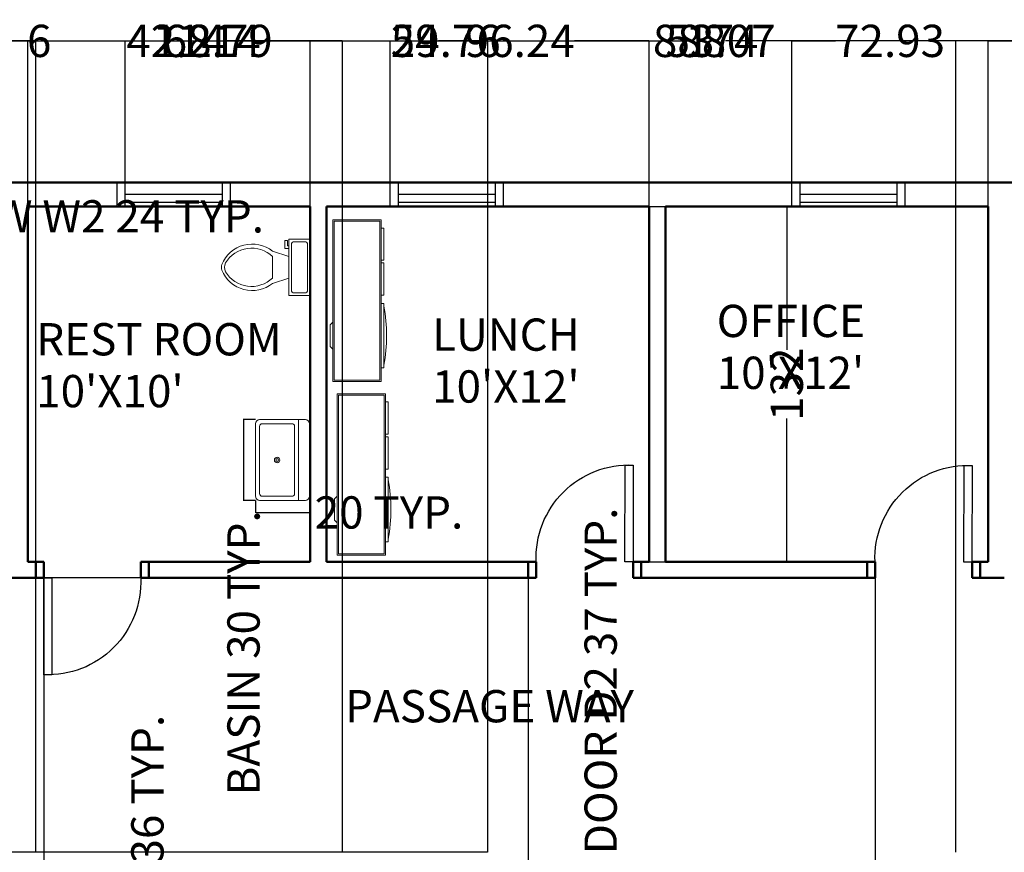
# Model space of a CAD drawing. Units: inches. Extents: x 128 to 1267, y -109 to 1208.
# Tile 3 of 8: x 418 to 784, y 194 to 503. Entities that reach past the tile are written whole.
import ezdxf

# ---------------------------------------------------------------- set-up
doc = ezdxf.new("R2010")
doc.units = ezdxf.units.IN
doc.header["$MEASUREMENT"] = 0
for name, color, linetype, lineweight in [('A-ANNO-DIMS', 2, 'Continuous', 18), ('A-AREA-IDEN', 3, 'Continuous', 25), ('A-DOOR', 4, 'Continuous', 25), ('A-FLOR-FIXT', 8, 'Continuous', 18), ('A-FURN', 8, 'Continuous', 18), ('A-GLAZ', 3, 'Continuous', 25), ('A-WALL', 7, 'Continuous', 50)]:
    doc.layers.add(name, color=color, linetype=linetype, lineweight=lineweight)
doc.styles.get("Standard").update_dxf_attribs({"font": 'arial.ttf'})
doc.dimstyles.get("Standard").update_dxf_attribs({"dimtxt": 12, "dimasz": 0.18, "dimexe": 0.18, "dimexo": 0.0625, "dimgap": 0.09, "dimtad": 0, "dimdec": 1, "dimzin": 0, "dimdsep": 46, "dimlunit": 3, "dimtxsty": 'Standard', "dimcen": 0.09, "dimadec": 0, "dimazin": 0, "dimtfac": 1, "dimtdec": 1, "dimtofl": 0, "dimtmove": 0, "dimatfit": 3, "dimfxl": 1, "dimtolj": 1, "dimtzin": 0, "dimarcsym": 0})

# ---------------------------------------------------------------- blocks, each defined once
blk = doc.blocks.new('Toilet - top')
for p, q in [((9.5, -6), (9.5, -2)), ((-10, -8.5), (-8, -8.5)), ((-10, -9.5), (-10, -8.5)), ((-7, -9.5), (-10, -9.5)), ((-8, -8.5), (-8, -8)), ((-7, -8), (-7, -9.5)), ((-4, -8), (-6, -14)), ((4, -8), (6, -14)), ((4, -14), (-4, -14))]:
    blk.add_line(p, q)
blk.add_lwpolyline([(10.5, -8), (10.5, 0), (-10.5, 0), (-10.5, -8)], close=True)
for points in [[(-9.5, -2), (-9.5, -6)], [(8.5, -1), (-8.5, -1)], [(-8.5, -7), (8.5, -7)]]:
    blk.add_lwpolyline(points)
for centre, radius, start, end in [((-8.62, -1.88), 0.884, 81.8699, 188.1301), ((8.62, -1.88), 0.884, 351.8699, 98.1301), ((-8.62, -6.12), 0.884, 171.8699, 278.1301), ((8.62, -6.12), 0.884, 261.8699, 8.1301), ((3.52, -21.58), 12.17, 141.4691, 247.9714), ((4.2, -21.82), 11.33, 136.3677, 238.9468), ((-3.52, -21.58), 12.17, 292.0284, 38.5307), ((-4.2, -21.82), 11.33, 301.053, 43.6321), ((0, -27.88), 4, 245.7318, 294.2682), ((0, -29), 4, 254.8605, 285.1395)]:
    blk.add_arc(centre, radius, start, end)
blk = doc.blocks.new('Entertainment Center')
for p, q in [((-4, 0), (-5, -1)), ((4, 0), (-4, 0)), ((5, -1), (4, 0)), ((-17, -19), (-17, -1)), ((-17, -1), (43, -1)), ((-16.5, -18.5), (-16.5, -1.5)), ((-16.5, -1.5), (42.5, -1.5)), ((42.5, -1.5), (42.5, -18.5)), ((43, -1), (43, -19)), ((43, -19), (-17, -19)), ((42.5, -18.5), (-16.5, -18.5)), ((-12, -20), (-12, -19)), ((12, -20), (-12, -20)), ((12, -19), (12, -20)), ((15, -20), (15, -19)), ((27, -20), (15, -20)), ((27, -19), (27, -20)), ((28, -20), (28, -19)), ((40, -20), (28, -20)), ((40, -19), (40, -20))]:
    blk.add_line(p, q)
blk.add_arc((0, 40), 61, 259.6111, 280.3889)
blk = doc.blocks.new('Sink-single - 30 in top')
blk.add_line((-15, -3.999996), (15, -3.999996))
for points in [[(-13.5, 0), (13.5, 0)], [(-15, -18.499996), (-15, -1.5)], [(15, -1.5), (15, -18.499996)], [(-13.5, -17.499996), (-13.5, -6.499996)], [(-12.5, -5.499996), (12.5, -5.499996)], [(13.5, -6.499996), (13.5, -17.499996)], [(13.5, -19.999996), (-13.5, -19.999996)], [(12.5, -18.499996), (-12.5, -18.499996)]]:
    blk.add_lwpolyline(points)
for radius in [1, 0.5]:
    blk.add_circle((0, -11.999996), radius)
for centre, radius, start, end in [((-13.5, -1.5), 1.5, 90, 180), ((13.5, -1.5), 1.5, 0, 90), ((-12.5, -6.499996), 1, 90, 180), ((12.5, -6.499996), 1, 0, 90), ((-12.5, -17.499996), 1, 180, 270), ((12.5, -17.499996), 1, 270, 0), ((-13.5, -18.499996), 1.5, 180, 270), ((13.5, -18.499996), 1.5, 270, 0)]:
    blk.add_arc(centre, radius, start, end)
blk = doc.blocks.new('DOOR-900')
blk.add_lwpolyline([(460.06, 187.64), (457.06, 187.64), (457.06, 151.64), (460.06, 151.64)], close=True)
blk.add_arc((458.56, 186.14), 34.53, 177.5104, 272.4896)
blk = doc.blocks.new('WIN-900')
for p, q in [((1102.06, 345.56), (1111.06, 345.56)), ((1102.06, 342.56), (1111.06, 342.56)), ((1103.56, 306.56), (1103.56, 342.56)), ((1106.56, 306.56), (1106.56, 342.56)), ((1111.06, 306.56), (1102.06, 306.56)), ((1111.06, 303.56), (1102.06, 303.56))]:
    blk.add_line(p, q)
blk = doc.blocks.new('*D11')
at = {"layer": 'A-ANNO-DIMS', "color": 0, "lineweight": -2, "transparency": 16777216}
for p, q in [((460.12, 187.64), (465.7, 187.64)), ((465.52, 187.64), (465.52, 187.82)), ((465.52, 151.4), (465.52, 187.46)), ((460.12, 151.22), (465.7, 151.22))]:
    blk.add_line(p, q, dxfattribs=at)
at = {"layer": 'A-ANNO-DIMS', "color": 0, "transparency": 16777216}
for points in [[(465.49, 187.46), (465.55, 187.46), (465.52, 187.64)], [(465.49, 151.4), (465.55, 151.4), (465.52, 151.22)]]:
    blk.add_solid(points, dxfattribs=at)
at = {"layer": 'Defpoints', "color": 0, "transparency": 16777216}
for p in [(460.06, 187.64), (465.52, 187.64), (460.06, 151.22)]:
    blk.add_point(p, dxfattribs=at)
at = {"layer": 'A-ANNO-DIMS', "color": 0, "transparency": 16777216, "insert": (465.52, 217.11), "char_height": 12, "attachment_point": 5, "rotation": 90}
blk.add_mtext('\\A1;36 TYP.', dxfattribs=at)
blk = doc.blocks.new('*D14')
at = {"layer": 'A-ANNO-DIMS', "color": 0, "lineweight": -2, "transparency": 16777216}
for p, q in [((323.73, 433.58), (323.73, 429.86)), ((347.73, 433.58), (347.73, 429.86)), ((323.91, 430.04), (347.55, 430.04)), ((347.73, 430.04), (347.91, 430.04))]:
    blk.add_line(p, q, dxfattribs=at)
at = {"layer": 'A-ANNO-DIMS', "color": 0, "transparency": 16777216}
for points in [[(323.91, 430.07), (323.91, 430.01), (323.73, 430.04)], [(347.55, 430.07), (347.55, 430.01), (347.73, 430.04)]]:
    blk.add_solid(points, dxfattribs=at)
at = {"layer": 'Defpoints', "color": 0, "transparency": 16777216}
for p in [(323.73, 433.64), (347.73, 433.64), (347.73, 430.04)]:
    blk.add_point(p, dxfattribs=at)
at = {"layer": 'A-ANNO-DIMS', "color": 0, "transparency": 16777216, "insert": (431.46, 430.04), "char_height": 12, "attachment_point": 5}
blk.add_mtext('\\A1;WINDOW W2 24 TYP.', dxfattribs=at)
blk = doc.blocks.new('*D18')
at = {"layer": 'A-ANNO-DIMS', "color": 0, "lineweight": -2, "transparency": 16777216}
for p, q in [((505.69, 354.47), (501.07, 354.47)), ((501.25, 354.29), (501.25, 324.65)), ((505.69, 324.47), (501.07, 324.47)), ((501.25, 324.47), (501.25, 324.29))]:
    blk.add_line(p, q, dxfattribs=at)
at = {"layer": 'A-ANNO-DIMS', "color": 0, "transparency": 16777216}
for points in [[(501.22, 354.29), (501.28, 354.29), (501.25, 354.47)], [(501.22, 324.65), (501.28, 324.65), (501.25, 324.47)]]:
    blk.add_solid(points, dxfattribs=at)
at = {"layer": 'Defpoints', "color": 0, "transparency": 16777216}
for p in [(505.75, 354.47), (501.25, 324.47), (505.75, 324.47)]:
    blk.add_point(p, dxfattribs=at)
at = {"layer": 'A-ANNO-DIMS', "color": 0, "transparency": 16777216, "insert": (501.25, 267.77), "char_height": 12, "attachment_point": 5, "rotation": 90}
blk.add_mtext('\\A1;BASIN 30 TYP.', dxfattribs=at)
blk = doc.blocks.new('*D19')
at = {"layer": 'A-ANNO-DIMS', "color": 0, "lineweight": -2, "transparency": 16777216}
for p, q in [((505.75, 324.4), (505.75, 319.79)), ((525.75, 324.4), (525.75, 319.79)), ((505.93, 319.97), (525.57, 319.97)), ((525.75, 319.97), (525.93, 319.97))]:
    blk.add_line(p, q, dxfattribs=at)
at = {"layer": 'A-ANNO-DIMS', "color": 0, "transparency": 16777216}
for points in [[(505.93, 320), (505.93, 319.94), (505.75, 319.97)], [(525.57, 320), (525.57, 319.94), (525.75, 319.97)]]:
    blk.add_solid(points, dxfattribs=at)
at = {"layer": 'Defpoints', "color": 0, "transparency": 16777216}
for p in [(505.75, 324.47), (525.75, 324.47), (525.75, 319.97)]:
    blk.add_point(p, dxfattribs=at)
at = {"layer": 'A-ANNO-DIMS', "color": 0, "transparency": 16777216, "insert": (555.33, 319.97), "char_height": 12, "attachment_point": 5}
blk.add_mtext('\\A1;20 TYP.', dxfattribs=at)
blk = doc.blocks.new('*D20')
at = {"layer": 'A-ANNO-DIMS', "color": 0, "lineweight": -2, "transparency": 16777216}
for p, q in [((628.59, 187.64), (634.19, 187.64)), ((634.01, 187.64), (634.01, 187.82)), ((634.01, 151.23), (634.01, 187.46)), ((628.59, 151.05), (634.19, 151.05))]:
    blk.add_line(p, q, dxfattribs=at)
at = {"layer": 'A-ANNO-DIMS', "color": 0, "transparency": 16777216}
for points in [[(633.98, 187.46), (634.04, 187.46), (634.01, 187.64)], [(633.98, 151.23), (634.04, 151.23), (634.01, 151.05)]]:
    blk.add_solid(points, dxfattribs=at)
at = {"layer": 'Defpoints', "color": 0, "transparency": 16777216}
for p in [(628.52, 187.64), (634.01, 187.64), (628.52, 151.05)]:
    blk.add_point(p, dxfattribs=at)
at = {"layer": 'A-ANNO-DIMS', "color": 0, "transparency": 16777216, "insert": (634.01, 257.34), "char_height": 12, "attachment_point": 5, "rotation": 90}
blk.add_mtext('\\A1;DOOR D2 37 TYP.', dxfattribs=at)
blk = doc.blocks.new('*D22')
at = {"layer": 'A-ANNO-DIMS', "color": 0, "lineweight": -2, "transparency": 16777216}
for p, q in [((223.06, -17.52), (223.06, 495.44)), ((223.24, 495.26), (653.69, 495.26)), ((1110.88, 495.26), (680.42, 495.26)), ((1111.06, -17.52), (1111.06, 495.44))]:
    blk.add_line(p, q, dxfattribs=at)
at = {"layer": 'A-ANNO-DIMS', "color": 0, "transparency": 16777216}
for points in [[(223.24, 495.29), (223.24, 495.23), (223.06, 495.26)], [(1110.88, 495.29), (1110.88, 495.23), (1111.06, 495.26)]]:
    blk.add_solid(points, dxfattribs=at)
at = {"layer": 'Defpoints', "color": 0, "transparency": 16777216}
for p in [(1111.06, 495.26), (223.06, -17.58), (1111.06, -17.58)]:
    blk.add_point(p, dxfattribs=at)
at = {"layer": 'A-ANNO-DIMS', "color": 0, "transparency": 16777216, "insert": (667.06, 495.26), "char_height": 12, "attachment_point": 5}
blk.add_mtext('\\A1;888', dxfattribs=at)
blk = doc.blocks.new('*D45')
at = {"layer": 'A-ANNO-DIMS', "color": 0, "lineweight": -2, "transparency": 16777216}
for p, q in [((415.06, 433.7), (415.06, 495.44)), ((415.24, 495.26), (457.09, 495.26)), ((457.27, 442.7), (457.27, 495.44)), ((457.27, 495.26), (457.45, 495.26))]:
    blk.add_line(p, q, dxfattribs=at)
at = {"layer": 'A-ANNO-DIMS', "color": 0, "transparency": 16777216}
for points in [[(415.24, 495.29), (415.24, 495.23), (415.06, 495.26)], [(457.09, 495.29), (457.09, 495.23), (457.27, 495.26)]]:
    blk.add_solid(points, dxfattribs=at)
at = {"layer": 'Defpoints', "color": 0, "transparency": 16777216}
for p in [(457.27, 495.26), (457.27, 442.64), (415.06, 433.64)]:
    blk.add_point(p, dxfattribs=at)
at = {"layer": 'A-ANNO-DIMS', "color": 0, "transparency": 16777216, "insert": (482.67, 495.26), "char_height": 12, "attachment_point": 5}
blk.add_mtext('\\A1;42.214', dxfattribs=at)
blk = doc.blocks.new('*D46')
at = {"layer": 'A-ANNO-DIMS', "color": 0, "lineweight": -2, "transparency": 16777216}
for p, q in [((457.27, 442.7), (457.27, 495.44)), ((457.45, 495.26), (471.28, 495.26)), ((525.88, 495.26), (512.05, 495.26)), ((526.06, 433.7), (526.06, 495.44))]:
    blk.add_line(p, q, dxfattribs=at)
at = {"layer": 'A-ANNO-DIMS', "color": 0, "transparency": 16777216}
for points in [[(457.45, 495.29), (457.45, 495.23), (457.27, 495.26)], [(525.88, 495.29), (525.88, 495.23), (526.06, 495.26)]]:
    blk.add_solid(points, dxfattribs=at)
at = {"layer": 'Defpoints', "color": 0, "transparency": 16777216}
for p in [(526.06, 495.26), (457.27, 442.64), (526.06, 433.64)]:
    blk.add_point(p, dxfattribs=at)
at = {"layer": 'A-ANNO-DIMS', "color": 0, "transparency": 16777216, "insert": (491.66, 495.26), "char_height": 12, "attachment_point": 5}
blk.add_mtext('\\A1;68.79', dxfattribs=at)
blk = doc.blocks.new('*D47')
at = {"layer": 'A-ANNO-DIMS', "color": 0, "lineweight": -2, "transparency": 16777216}
for p, q in [((526.06, 433.7), (526.06, 495.44)), ((526.24, 495.26), (555.64, 495.26)), ((555.82, 442.7), (555.82, 495.44)), ((555.82, 495.26), (556, 495.26))]:
    blk.add_line(p, q, dxfattribs=at)
at = {"layer": 'A-ANNO-DIMS', "color": 0, "transparency": 16777216}
for points in [[(526.24, 495.29), (526.24, 495.23), (526.06, 495.26)], [(555.64, 495.29), (555.64, 495.23), (555.82, 495.26)]]:
    blk.add_solid(points, dxfattribs=at)
at = {"layer": 'Defpoints', "color": 0, "transparency": 16777216}
for p in [(555.82, 495.26), (555.82, 442.64), (526.06, 433.64)]:
    blk.add_point(p, dxfattribs=at)
at = {"layer": 'A-ANNO-DIMS', "color": 0, "transparency": 16777216, "insert": (576.43, 495.26), "char_height": 12, "attachment_point": 5}
blk.add_mtext('\\A1;29.76', dxfattribs=at)
blk = doc.blocks.new('*D48')
at = {"layer": 'A-ANNO-DIMS', "color": 0, "lineweight": -2, "transparency": 16777216}
for p, q in [((555.82, 442.7), (555.82, 495.44)), ((556, 495.26), (583.62, 495.26)), ((651.88, 495.26), (624.25, 495.26)), ((652.06, 433.7), (652.06, 495.44))]:
    blk.add_line(p, q, dxfattribs=at)
at = {"layer": 'A-ANNO-DIMS', "color": 0, "transparency": 16777216}
for points in [[(556, 495.29), (556, 495.23), (555.82, 495.26)], [(651.88, 495.29), (651.88, 495.23), (652.06, 495.26)]]:
    blk.add_solid(points, dxfattribs=at)
at = {"layer": 'Defpoints', "color": 0, "transparency": 16777216}
for p in [(652.06, 495.26), (555.82, 442.64), (652.06, 433.64)]:
    blk.add_point(p, dxfattribs=at)
at = {"layer": 'A-ANNO-DIMS', "color": 0, "transparency": 16777216, "insert": (603.94, 495.26), "char_height": 12, "attachment_point": 5}
blk.add_mtext('\\A1;96.24', dxfattribs=at)
blk = doc.blocks.new('*D49')
at = {"layer": 'A-ANNO-DIMS', "color": 0, "lineweight": -2, "transparency": 16777216}
for p, q in [((652.06, 433.7), (652.06, 495.44)), ((652.24, 495.26), (658.25, 495.26)), ((704.95, 495.26), (698.93, 495.26)), ((705.13, 442.7), (705.13, 495.44))]:
    blk.add_line(p, q, dxfattribs=at)
at = {"layer": 'A-ANNO-DIMS', "color": 0, "transparency": 16777216}
for points in [[(652.24, 495.29), (652.24, 495.23), (652.06, 495.26)], [(704.95, 495.29), (704.95, 495.23), (705.13, 495.26)]]:
    blk.add_solid(points, dxfattribs=at)
at = {"layer": 'Defpoints', "color": 0, "transparency": 16777216}
for p in [(705.13, 495.26), (705.13, 442.64), (652.06, 433.64)]:
    blk.add_point(p, dxfattribs=at)
at = {"layer": 'A-ANNO-DIMS', "color": 0, "transparency": 16777216, "insert": (678.59, 495.26), "char_height": 12, "attachment_point": 5}
blk.add_mtext('\\A1;53.07', dxfattribs=at)
blk = doc.blocks.new('*D50')
at = {"layer": 'A-ANNO-DIMS', "color": 0, "lineweight": -2, "transparency": 16777216}
for p, q in [((705.13, 442.7), (705.13, 495.44)), ((705.31, 495.26), (721.3, 495.26)), ((777.88, 495.26), (761.88, 495.26)), ((778.06, 433.7), (778.06, 495.44))]:
    blk.add_line(p, q, dxfattribs=at)
at = {"layer": 'A-ANNO-DIMS', "color": 0, "transparency": 16777216}
for points in [[(705.31, 495.29), (705.31, 495.23), (705.13, 495.26)], [(777.88, 495.29), (777.88, 495.23), (778.06, 495.26)]]:
    blk.add_solid(points, dxfattribs=at)
at = {"layer": 'Defpoints', "color": 0, "transparency": 16777216}
for p in [(778.06, 495.26), (705.13, 442.64), (778.06, 433.64)]:
    blk.add_point(p, dxfattribs=at)
at = {"layer": 'A-ANNO-DIMS', "color": 0, "transparency": 16777216, "insert": (741.59, 495.26), "char_height": 12, "attachment_point": 5}
blk.add_mtext('\\A1;72.93', dxfattribs=at)
blk = doc.blocks.new('*D51')
at = {"layer": 'A-ANNO-DIMS', "color": 0, "lineweight": -2, "transparency": 16777216}
for p, q in [((778.06, 433.7), (778.06, 495.44)), ((778.24, 495.26), (794, 495.26)), ((794.18, 442.7), (794.18, 495.44)), ((794.18, 495.26), (794.36, 495.26))]:
    blk.add_line(p, q, dxfattribs=at)
at = {"layer": 'A-ANNO-DIMS', "color": 0, "transparency": 16777216}
for points in [[(778.24, 495.29), (778.24, 495.23), (778.06, 495.26)], [(794, 495.29), (794, 495.23), (794.18, 495.26)]]:
    blk.add_solid(points, dxfattribs=at)
at = {"layer": 'Defpoints', "color": 0, "transparency": 16777216}
for p in [(794.18, 495.26), (794.18, 442.64), (778.06, 433.64)]:
    blk.add_point(p, dxfattribs=at)
at = {"layer": 'A-ANNO-DIMS', "color": 0, "transparency": 16777216, "insert": (814.07, 495.26), "char_height": 12, "attachment_point": 5}
blk.add_mtext('\\A1;16.12', dxfattribs=at)
blk = doc.blocks.new('*D66')
at = {"layer": 'A-ANNO-DIMS', "color": 0, "lineweight": -2, "transparency": 16777216}
for p, q in [((415.06, 433.7), (415.06, 495.44)), ((415.24, 495.26), (420.88, 495.26)), ((421.06, 433.7), (421.06, 495.44)), ((421.06, 495.26), (421.24, 495.26))]:
    blk.add_line(p, q, dxfattribs=at)
at = {"layer": 'A-ANNO-DIMS', "color": 0, "transparency": 16777216}
for points in [[(415.24, 495.29), (415.24, 495.23), (415.06, 495.26)], [(420.88, 495.29), (420.88, 495.23), (421.06, 495.26)]]:
    blk.add_solid(points, dxfattribs=at)
at = {"layer": 'Defpoints', "color": 0, "transparency": 16777216}
for p in [(421.06, 495.26), (415.06, 433.64), (421.06, 433.64)]:
    blk.add_point(p, dxfattribs=at)
at = {"layer": 'A-ANNO-DIMS', "color": 0, "transparency": 16777216, "insert": (425.29, 495.26), "char_height": 12, "attachment_point": 5}
blk.add_mtext('\\A1;6', dxfattribs=at)
blk = doc.blocks.new('*D73')
at = {"layer": 'A-ANNO-DIMS', "color": 0, "lineweight": -2, "transparency": 16777216}
for p, q in [((652.12, 433.64), (703.39, 433.64)), ((703.21, 433.46), (703.21, 380.36)), ((703.21, 301.82), (703.21, 354.92)), ((652.12, 301.64), (703.39, 301.64))]:
    blk.add_line(p, q, dxfattribs=at)
at = {"layer": 'A-ANNO-DIMS', "color": 0, "transparency": 16777216}
for points in [[(703.18, 433.46), (703.24, 433.46), (703.21, 433.64)], [(703.18, 301.82), (703.24, 301.82), (703.21, 301.64)]]:
    blk.add_solid(points, dxfattribs=at)
at = {"layer": 'Defpoints', "color": 0, "transparency": 16777216}
for p in [(652.06, 433.64), (652.06, 301.64), (703.21, 301.64)]:
    blk.add_point(p, dxfattribs=at)
at = {"layer": 'A-ANNO-DIMS', "color": 0, "transparency": 16777216, "insert": (703.21, 367.64), "char_height": 12, "attachment_point": 5, "rotation": 90}
blk.add_mtext('\\A1;132', dxfattribs=at)
blk = doc.blocks.new('*D74')
at = {"layer": 'A-ANNO-DIMS', "color": 0, "lineweight": -2, "transparency": 16777216}
for p, q in [((606.99, 295.64), (135.73, 295.64)), ((135.91, 295.46), (135.91, 257.36)), ((135.91, 193.82), (135.91, 231.92)), ((591.99, 193.64), (135.73, 193.64))]:
    blk.add_line(p, q, dxfattribs=at)
at = {"layer": 'A-ANNO-DIMS', "color": 0, "transparency": 16777216}
for points in [[(135.88, 295.46), (135.94, 295.46), (135.91, 295.64)], [(135.88, 193.82), (135.94, 193.82), (135.91, 193.64)]]:
    blk.add_solid(points, dxfattribs=at)
at = {"layer": 'Defpoints', "color": 0, "transparency": 16777216}
for p in [(607.06, 295.64), (135.91, 193.64), (592.06, 193.64)]:
    blk.add_point(p, dxfattribs=at)
at = {"layer": 'A-ANNO-DIMS', "color": 0, "transparency": 16777216, "insert": (135.91, 244.64), "char_height": 12, "attachment_point": 5, "rotation": 90}
blk.add_mtext('\\A1;102', dxfattribs=at)
blk = doc.blocks.new('*D76')
at = {"layer": 'A-ANNO-DIMS', "color": 0, "lineweight": -2, "transparency": 16777216}
for p, q in [((373.06, 295.58), (373.06, -82.19)), ((427.06, 295.58), (427.06, -82.19)), ((373.24, -82.01), (391.4, -82.01)), ((426.88, -82.01), (408.72, -82.01))]:
    blk.add_line(p, q, dxfattribs=at)
at = {"layer": 'A-ANNO-DIMS', "color": 0, "transparency": 16777216}
for points in [[(373.24, -81.98), (373.24, -82.04), (373.06, -82.01)], [(426.88, -81.98), (426.88, -82.04), (427.06, -82.01)]]:
    blk.add_solid(points, dxfattribs=at)
at = {"layer": 'Defpoints', "color": 0, "transparency": 16777216}
for p in [(373.06, 295.64), (427.06, 295.64), (427.06, -82.01)]:
    blk.add_point(p, dxfattribs=at)
at = {"layer": 'A-ANNO-DIMS', "color": 0, "transparency": 16777216, "insert": (400.06, -82.01), "char_height": 12, "attachment_point": 5}
blk.add_mtext('\\A1;54', dxfattribs=at)
blk = doc.blocks.new('*D77')
at = {"layer": 'A-ANNO-DIMS', "color": 0, "lineweight": -2, "transparency": 16777216}
for p, q in [((427.06, 295.58), (427.06, -82.19)), ((607.06, 295.58), (607.06, -82.19)), ((427.24, -82.01), (504.29, -82.01)), ((606.88, -82.01), (529.82, -82.01))]:
    blk.add_line(p, q, dxfattribs=at)
at = {"layer": 'A-ANNO-DIMS', "color": 0, "transparency": 16777216}
for points in [[(427.24, -81.98), (427.24, -82.04), (427.06, -82.01)], [(606.88, -81.98), (606.88, -82.04), (607.06, -82.01)]]:
    blk.add_solid(points, dxfattribs=at)
at = {"layer": 'Defpoints', "color": 0, "transparency": 16777216}
for p in [(427.06, 295.64), (607.06, 295.64), (607.06, -82.01)]:
    blk.add_point(p, dxfattribs=at)
at = {"layer": 'A-ANNO-DIMS', "color": 0, "transparency": 16777216, "insert": (517.06, -82.01), "char_height": 12, "attachment_point": 5}
blk.add_mtext('\\A1;180', dxfattribs=at)
blk = doc.blocks.new('*D78')
at = {"layer": 'A-ANNO-DIMS', "color": 0, "lineweight": -2, "transparency": 16777216}
for p, q in [((607.06, 295.58), (607.06, -82.19)), ((736.06, 295.58), (736.06, -82.19)), ((607.24, -82.01), (658.76, -82.01)), ((735.88, -82.01), (684.35, -82.01))]:
    blk.add_line(p, q, dxfattribs=at)
at = {"layer": 'A-ANNO-DIMS', "color": 0, "transparency": 16777216}
for points in [[(607.24, -81.98), (607.24, -82.04), (607.06, -82.01)], [(735.88, -81.98), (735.88, -82.04), (736.06, -82.01)]]:
    blk.add_solid(points, dxfattribs=at)
at = {"layer": 'Defpoints', "color": 0, "transparency": 16777216}
for p in [(607.06, 295.64), (736.06, 295.64), (736.06, -82.01)]:
    blk.add_point(p, dxfattribs=at)
at = {"layer": 'A-ANNO-DIMS', "color": 0, "transparency": 16777216, "insert": (671.56, -82.01), "char_height": 12, "attachment_point": 5}
blk.add_mtext('\\A1;129', dxfattribs=at)
blk = doc.blocks.new('*D79')
at = {"layer": 'A-ANNO-DIMS', "color": 0, "lineweight": -2, "transparency": 16777216}
for p, q in [((313.06, 193.7), (313.06, 495.44)), ((313.24, 495.26), (356.93, 495.26)), ((423.88, 495.26), (380.18, 495.26)), ((424.06, 193.7), (424.06, 495.44))]:
    blk.add_line(p, q, dxfattribs=at)
at = {"layer": 'A-ANNO-DIMS', "color": 0, "transparency": 16777216}
for points in [[(313.24, 495.29), (313.24, 495.23), (313.06, 495.26)], [(423.88, 495.29), (423.88, 495.23), (424.06, 495.26)]]:
    blk.add_solid(points, dxfattribs=at)
at = {"layer": 'Defpoints', "color": 0, "transparency": 16777216}
for p in [(424.06, 495.26), (313.06, 193.64), (424.06, 193.64)]:
    blk.add_point(p, dxfattribs=at)
at = {"layer": 'A-ANNO-DIMS', "color": 0, "transparency": 16777216, "insert": (368.56, 495.26), "char_height": 12, "attachment_point": 5}
blk.add_mtext('\\A1;111', dxfattribs=at)
blk = doc.blocks.new('*D80')
at = {"layer": 'A-ANNO-DIMS', "color": 0, "lineweight": -2, "transparency": 16777216}
for p, q in [((424.06, 193.7), (424.06, 495.44)), ((424.24, 495.26), (468.3, 495.26)), ((537.88, 495.26), (493.81, 495.26)), ((538.06, 193.7), (538.06, 495.44))]:
    blk.add_line(p, q, dxfattribs=at)
at = {"layer": 'A-ANNO-DIMS', "color": 0, "transparency": 16777216}
for points in [[(424.24, 495.29), (424.24, 495.23), (424.06, 495.26)], [(537.88, 495.29), (537.88, 495.23), (538.06, 495.26)]]:
    blk.add_solid(points, dxfattribs=at)
at = {"layer": 'Defpoints', "color": 0, "transparency": 16777216}
for p in [(538.06, 495.26), (424.06, 193.64), (538.06, 193.64)]:
    blk.add_point(p, dxfattribs=at)
at = {"layer": 'A-ANNO-DIMS', "color": 0, "transparency": 16777216, "insert": (481.06, 495.26), "char_height": 12, "attachment_point": 5}
blk.add_mtext('\\A1;114', dxfattribs=at)
blk = doc.blocks.new('*D81')
at = {"layer": 'A-ANNO-DIMS', "color": 0, "lineweight": -2, "transparency": 16777216}
for p, q in [((538.06, 193.7), (538.06, 495.44)), ((538.24, 495.26), (556.4, 495.26)), ((591.88, 495.26), (573.72, 495.26)), ((592.06, 193.7), (592.06, 495.44))]:
    blk.add_line(p, q, dxfattribs=at)
at = {"layer": 'A-ANNO-DIMS', "color": 0, "transparency": 16777216}
for points in [[(538.24, 495.29), (538.24, 495.23), (538.06, 495.26)], [(591.88, 495.29), (591.88, 495.23), (592.06, 495.26)]]:
    blk.add_solid(points, dxfattribs=at)
at = {"layer": 'Defpoints', "color": 0, "transparency": 16777216}
for p in [(592.06, 495.26), (538.06, 193.64), (592.06, 193.64)]:
    blk.add_point(p, dxfattribs=at)
at = {"layer": 'A-ANNO-DIMS', "color": 0, "transparency": 16777216, "insert": (565.06, 495.26), "char_height": 12, "attachment_point": 5}
blk.add_mtext('\\A1;54', dxfattribs=at)
blk = doc.blocks.new('*D82')
at = {"layer": 'A-ANNO-DIMS', "color": 0, "lineweight": -2, "transparency": 16777216}
for p, q in [((592.06, 193.7), (592.06, 495.44)), ((592.24, 495.26), (666.3, 495.26)), ((765.88, 495.26), (691.81, 495.26)), ((766.06, 193.7), (766.06, 495.44))]:
    blk.add_line(p, q, dxfattribs=at)
at = {"layer": 'A-ANNO-DIMS', "color": 0, "transparency": 16777216}
for points in [[(592.24, 495.29), (592.24, 495.23), (592.06, 495.26)], [(765.88, 495.29), (765.88, 495.23), (766.06, 495.26)]]:
    blk.add_solid(points, dxfattribs=at)
at = {"layer": 'Defpoints', "color": 0, "transparency": 16777216}
for p in [(766.06, 495.26), (592.06, 193.64), (766.06, 193.64)]:
    blk.add_point(p, dxfattribs=at)
at = {"layer": 'A-ANNO-DIMS', "color": 0, "transparency": 16777216, "insert": (679.06, 495.26), "char_height": 12, "attachment_point": 5}
blk.add_mtext('\\A1;174', dxfattribs=at)

msp = doc.modelspace()

# ---------------------------------------------------------------- linework, layer by layer
at = {"layer": 'A-WALL'}
for p, q in [((526.056, 433.6399), (421.056, 433.6399)), ((421.056, 433.6399), (421.056, 301.6399)), ((526.056, 301.6399), (526.056, 433.6399)), ((532.056, 301.6399), (532.056, 433.6399)), ((652.056, 433.6399), (532.056, 433.6399)), ((652.056, 301.6399), (652.056, 433.6399)), ((658.056, 301.6399), (658.056, 433.6399)), ((778.056, 433.6399), (658.056, 433.6399)), ((778.056, 301.6399), (778.056, 433.6399)), ((427.056, 301.6399), (421.056, 301.6399)), ((424.056, 301.6399), (424.056, 295.6399)), ((427.056, 301.6399), (427.056, 295.6399)), ((526.056, 301.6399), (463.056, 301.6399)), ((463.056, 301.6399), (463.056, 295.6399)), ((466.056, 301.6399), (466.056, 295.6399)), ((610.056, 301.6399), (532.056, 301.6399)), ((607.056, 301.6399), (607.056, 295.6399)), ((610.056, 301.6399), (610.056, 295.6399)), ((652.056, 301.6399), (646.056, 301.6399)), ((646.056, 301.6399), (646.056, 295.6399)), ((649.056, 301.6399), (649.056, 295.6399)), ((736.056, 301.6399), (658.056, 301.6399)), ((733.056, 301.6399), (733.056, 295.6399)), ((736.056, 301.6399), (736.056, 295.6399)), ((778.056, 301.6399), (772.056, 301.6399)), ((772.056, 301.6399), (772.056, 295.6399)), ((775.056, 301.6399), (775.056, 295.6399)), ((427.056, 295.6399), (409.056, 295.6399)), ((532.056, 295.6399), (463.056, 295.6399)), ((610.056, 295.6399), (532.056, 295.6399)), ((658.056, 295.6399), (646.056, 295.6399)), ((736.056, 295.6399), (658.056, 295.6399)), ((784.056, 295.6399), (772.056, 295.6399))]:
    msp.add_line(p, q, dxfattribs=at)
msp.add_lwpolyline([(1111.056, 427.6399), (1111.056, 442.6399), (409.056, 442.6399)], dxfattribs=at)

# ---------------------------------------------------------------- block references
at = {"layer": 'A-DOOR', "extrusion": (0, 0, -1), "zscale": -1}
for p, rotation in [((-186.1618, 489.6681), 180.0532357876791), ((-312.8015, 491.1927), 180.2624381170907)]:
    msp.add_blockref('DOOR-900', p, dxfattribs=dict(at, rotation=rotation))
msp.add_blockref('DOOR-900', (-887.112, 108), dxfattribs=at)
at = {"layer": 'A-FLOR-FIXT', "rotation": 270}
for name, p in [('Toilet - top', (526.056, 411.0992)), ('Sink-single - 30 in top', (525.7546, 339.4664))]:
    msp.add_blockref(name, p, dxfattribs=at)
at = {"layer": 'A-FURN', "rotation": 90}
for p in [(533.4271, 385.6952), (535.0751, 321.0732)]:
    msp.add_blockref('Entertainment Center', p, dxfattribs=at)
at = {"layer": 'A-GLAZ'}
for p, rotation in [((799.8327, -668.4161), 90.00000000000036), ((901.378, -668.4161), 90.00000000000044), ((1050.688, -668.4161), 90.0000000000003)]:
    msp.add_blockref('WIN-900', p, dxfattribs=dict(at, rotation=rotation))

# ---------------------------------------------------------------- texts
at = {"layer": 'A-AREA-IDEN'}
for s, p in [('OFFICE', (677.1597, 385.1547)), ('LUNCH', (571.3689, 380.0706)), ('REST ROOM ', (424.1971, 378.3496)), ("10'X12'", (677.1597, 365.8777)), ("10'X12'", (571.3689, 360.7937)), ("10'X10'", (424.1971, 359.0727)), ('PASSAGE WAY', (539.0065, 241.9488))]:
    msp.add_text(s, height=12, dxfattribs=at).set_placement(p)

# ---------------------------------------------------------------- dimensions: what is measured, and where the dimension line sits
at = {"layer": 'A-ANNO-DIMS'}
for base, p1, p2, override, picture, middle in [((1111.056, 495.2611), (223.056, -17.5809), (1111.056, -17.5809), {"dimdec": 0, "dimlfac": 1, "dimrnd": 0, "dimzin": 0, "dimdsep": 46, "dimlunit": 2}, '*D22', (667.056, 495.2611)), ((424.056, 495.2611), (313.056, 193.6399), (424.056, 193.6399), {"dimdec": 0, "dimlfac": 1, "dimrnd": 0, "dimzin": 0, "dimdsep": 46, "dimlunit": 2}, '*D79', (368.556, 495.2611)), ((457.2704, 495.2611), (415.056, 433.6399), (457.2704, 442.6399), {"dimdec": 3, "dimlfac": 1, "dimrnd": 0, "dimzin": 0, "dimdsep": 46, "dimlunit": 2}, '*D45', (482.6659, 495.2611)), ((421.056, 495.2611), (415.056, 433.6399), (421.056, 433.6399), {"dimdec": 0, "dimlfac": 1, "dimrnd": 0, "dimzin": 0, "dimdsep": 46, "dimlunit": 2}, '*D66', (425.2878, 495.2611)), ((538.056, 495.2611), (424.056, 193.6399), (538.056, 193.6399), {"dimdec": 0, "dimlfac": 1, "dimrnd": 0, "dimzin": 0, "dimdsep": 46, "dimlunit": 2}, '*D80', (481.056, 495.2611)), ((526.056, 495.2611), (457.2704, 442.6399), (526.056, 433.6399), {"dimdec": 2, "dimlfac": 1, "dimrnd": 0, "dimzin": 0, "dimdsep": 46, "dimlunit": 2}, '*D46', (491.6632, 495.2611)), ((555.8157, 495.2611), (526.056, 433.6399), (555.8157, 442.6399), {"dimdec": 2, "dimlfac": 1, "dimrnd": 0, "dimzin": 0, "dimdsep": 46, "dimlunit": 2}, '*D47', (576.4308, 495.2611)), ((592.056, 495.2611), (538.056, 193.6399), (592.056, 193.6399), {"dimdec": 0, "dimlfac": 1, "dimrnd": 0, "dimzin": 0, "dimdsep": 46, "dimlunit": 2}, '*D81', (565.056, 495.2611)), ((652.056, 495.2611), (555.8157, 442.6399), (652.056, 433.6399), {"dimdec": 2, "dimlfac": 1, "dimrnd": 0, "dimzin": 0, "dimdsep": 46, "dimlunit": 2}, '*D48', (603.9358, 495.2611)), ((766.056, 495.2611), (592.056, 193.6399), (766.056, 193.6399), {"dimdec": 0, "dimlfac": 1, "dimrnd": 0, "dimzin": 0, "dimdsep": 46, "dimlunit": 2}, '*D82', (679.056, 495.2611)), ((705.1257, 495.2611), (652.056, 433.6399), (705.1257, 442.6399), {"dimdec": 2, "dimlfac": 1, "dimrnd": 0, "dimzin": 0, "dimdsep": 46, "dimlunit": 2}, '*D49', (678.5909, 495.2611)), ((778.056, 495.2611), (705.1257, 442.6399), (778.056, 433.6399), {"dimdec": 2, "dimlfac": 1, "dimrnd": 0, "dimzin": 0, "dimdsep": 46, "dimlunit": 2}, '*D50', (741.5909, 495.2611)), ((794.177, 495.2611), (778.056, 433.6399), (794.177, 442.6399), {"dimdec": 2, "dimlfac": 1, "dimrnd": 0, "dimzin": 0, "dimdsep": 46, "dimlunit": 2}, '*D51', (814.0677, 495.2611)), ((427.056, -82.0098), (373.056, 295.6399), (427.056, 295.6399), {"dimdec": 0, "dimlfac": 1, "dimrnd": 0, "dimzin": 0, "dimdsep": 46, "dimlunit": 2}, '*D76', (400.056, -82.0098)), ((607.056, -82.0098), (427.056, 295.6399), (607.056, 295.6399), {"dimdec": 0, "dimlfac": 1, "dimrnd": 0, "dimzin": 0, "dimdsep": 46, "dimlunit": 2}, '*D77', (517.056, -82.0098)), ((736.056, -82.0098), (607.056, 295.6399), (736.056, 295.6399), {"dimdec": 0, "dimlfac": 1, "dimrnd": 0, "dimzin": 0, "dimdsep": 46, "dimlunit": 2}, '*D78', (671.556, -82.0098))]:
    dim = msp.add_linear_dim(base=base, p1=p1, p2=p2, dimstyle='Standard', override=override, dxfattribs=at)
    dim.commit()
    dim.dimension.update_dxf_attribs({"geometry": picture, "text_midpoint": middle})
for base, p1, p2, text, picture, middle in [((347.73, 430.0399), (323.73, 433.6399), (347.73, 433.6399), 'WINDOW W2 <> TYP.', '*D14', (431.4598, 430.0399)), ((525.7546, 319.9664), (505.7546, 324.4664), (525.7546, 324.4664), '<> TYP.', '*D19', (555.333, 319.9664))]:
    dim = msp.add_linear_dim(base=base, p1=p1, p2=p2, text=text, dimstyle='Standard', override={"dimdec": 0, "dimrnd": 0, "dimzin": 0, "dimlunit": 2}, dxfattribs=at)
    dim.commit()
    dim.dimension.update_dxf_attribs({"geometry": picture, "text_midpoint": middle})
for base, p1, p2, angle, picture, middle in [((703.206, 301.6399), (652.056, 433.6399), (652.056, 301.6399), 270, '*D73', (703.206, 367.6399)), ((135.906, 193.6399), (607.056, 295.6399), (592.056, 193.6399), 90, '*D74', (135.906, 244.6399))]:
    dim = msp.add_linear_dim(base=base, p1=p1, p2=p2, angle=angle, dimstyle='Standard', override={"dimdec": 0, "dimlfac": 1, "dimrnd": 0, "dimzin": 0, "dimdsep": 46, "dimlunit": 2}, dxfattribs=at)
    dim.commit()
    dim.dimension.update_dxf_attribs({"geometry": picture, "text_midpoint": middle})
for base, p1, p2, angle, text, picture, middle in [((501.2546, 324.4664), (505.7546, 354.4664), (505.7546, 324.4664), 270, 'BASIN <> TYP.', '*D18', (501.2546, 267.7734)), ((634.0127, 187.6399), (628.5237, 151.0471), (628.5237, 187.6399), 90, 'DOOR D2 <> TYP.', '*D20', (634.0127, 257.3356)), ((465.5191, 187.6399), (460.056, 151.2195), (460.056, 187.6399), 90, '<> TYP.', '*D11', (465.5191, 217.1118))]:
    dim = msp.add_linear_dim(base=base, p1=p1, p2=p2, angle=angle, text=text, dimstyle='Standard', override={"dimdec": 0, "dimrnd": 0, "dimzin": 0, "dimlunit": 2}, dxfattribs=at)
    dim.commit()
    dim.dimension.update_dxf_attribs({"geometry": picture, "text_midpoint": middle})

doc.saveas('drawing.dxf')
